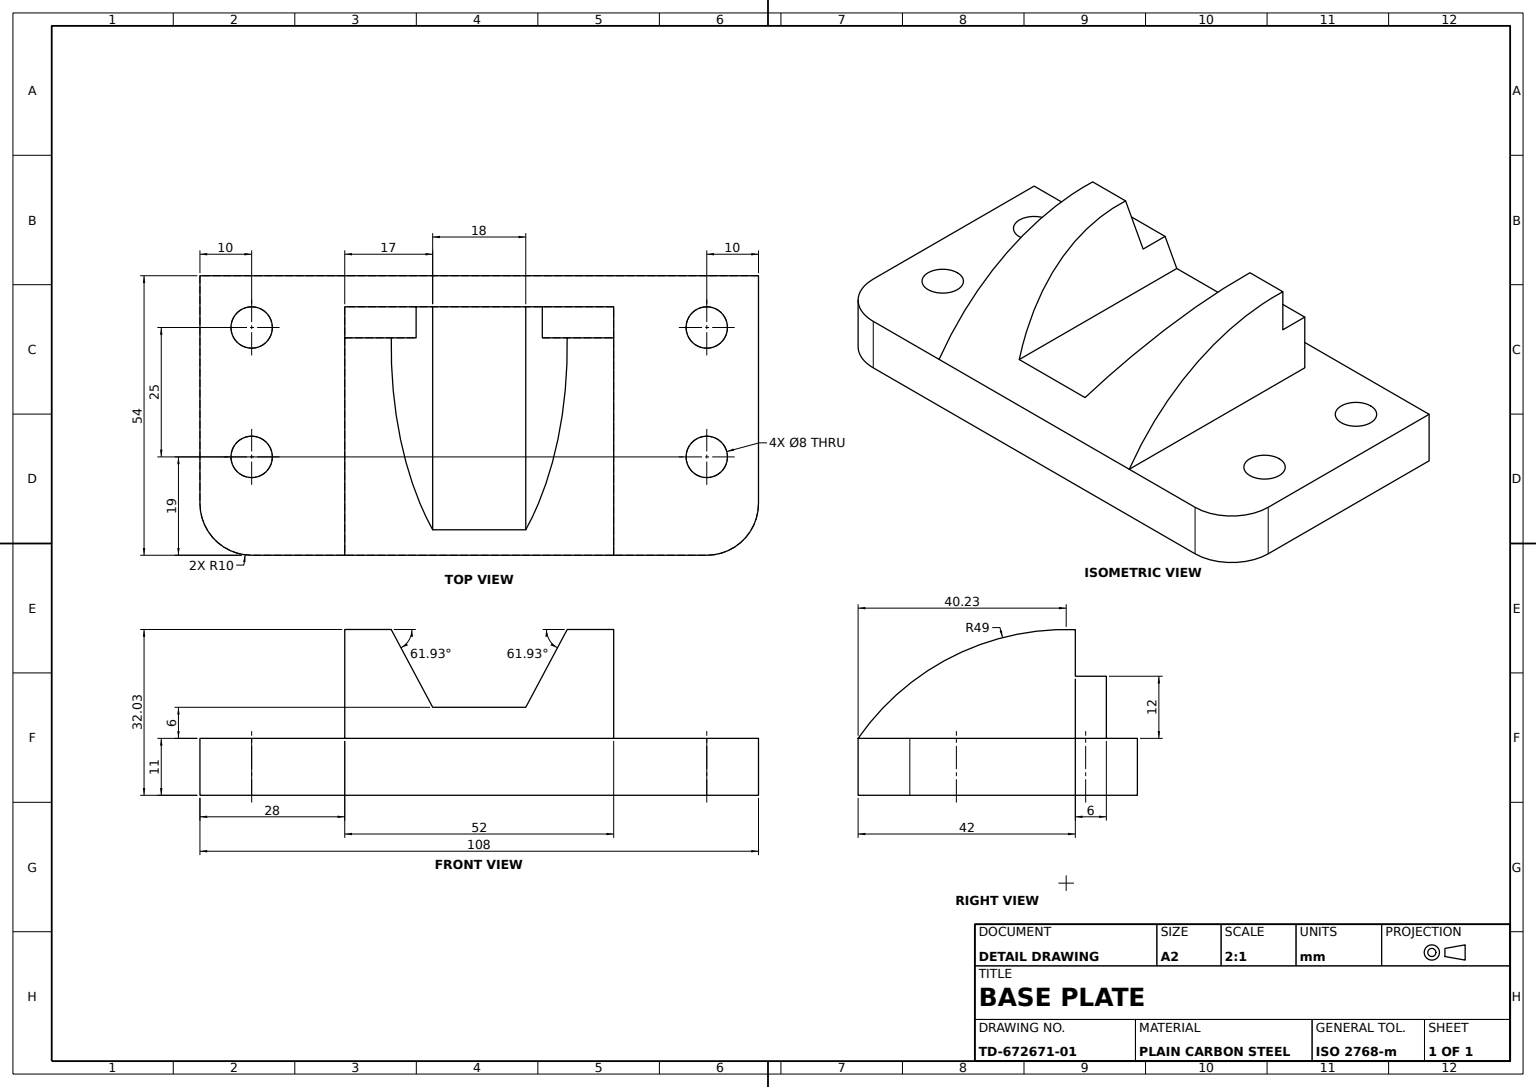
from build123d import *

# Parameters (mm, degrees)
BASE_PLATE_SKETCH_R          = 4
BASE_PLATE_DEPTH             = 11
SADDLE_BLOCK_SKETCH_W        = 52
SADDLE_BLOCK_SKETCH_H        = 48
SADDLE_BLOCK_DEPTH           = 61
SADDLE_ARC_PROFILE_CUT_DEPTH = 61
SADDLE_RELIEF_CUT_DEPTH      = 61


with BuildPart() as part:
    # Base Plate Sketch → Base Plate (new body)
    with BuildSketch(Plane(origin=(0, 0, 0), x_dir=(1, 0, 0), z_dir=(0, 1, 0))):
        with BuildLine():
            Line((-44, -27), (44, -27))
            ThreePointArc((44, -27), (51.071067812, -24.071067812), (54, -17))
            Line((54, -17), (54, 27))
            Line((54, 27), (-54, 27))
            Line((-54, 27), (-54, -17))
            ThreePointArc((-54, -17), (-51.071067812, -24.071067812), (-44, -27))
        make_face()
        with Locations(Location((-44, 17, 0), (0, 0, 270))):
            Circle(BASE_PLATE_SKETCH_R, mode=Mode.SUBTRACT)
        with Locations(Location((-44, -8, 0), (0, 0, 270))):
            Circle(BASE_PLATE_SKETCH_R, mode=Mode.SUBTRACT)
        with Locations(Location((44, 17, 0), (0, 0, 270))):
            Circle(BASE_PLATE_SKETCH_R, mode=Mode.SUBTRACT)
        with Locations(Location((44, -8, 0), (0, 0, 270))):
            Circle(BASE_PLATE_SKETCH_R, mode=Mode.SUBTRACT)
    extrude(amount=BASE_PLATE_DEPTH)

    # Saddle Block Sketch → Saddle Block (add)
    with BuildSketch(Plane(origin=(0, 11, 0), x_dir=(1, 0, 0), z_dir=(0, 1, 0))):
        with Locations((0, -3)):
            Rectangle(SADDLE_BLOCK_SKETCH_W, SADDLE_BLOCK_SKETCH_H)
    extrude(amount=SADDLE_BLOCK_DEPTH)

    # Saddle Arc Profile Sketch → Saddle Arc Profile Cut (cut)
    with BuildSketch(Plane(origin=(26, 0, 0), x_dir=(0, 0, -1), z_dir=(1, 0, 0))):
        with BuildLine():
            Line((15, 23), (15, 32))
            ThreePointArc((15, 32), (-8.67938185, 26.8587637), (-27, 11))
            Line((-27, 11), (-38.885663345, 11))
            Line((-38.885663345, 11), (-38.885663345, 85.95954857))
            Line((-38.885663345, 85.95954857), (45.449794115, 85.95954857))
            Line((45.449794115, 85.95954857), (44.243086456, 28.305738224))
            Line((44.243086456, 28.305738224), (21, 23))
            Line((21, 23), (15, 23))
        make_face()
    extrude(amount=-SADDLE_ARC_PROFILE_CUT_DEPTH, mode=Mode.SUBTRACT)

    # Saddle Relief Sketch → Saddle Relief Cut (cut)
    with BuildSketch(Plane.XY.offset(27)):
        Polygon((-17.016976715, 32.031831341), (17.016976715, 32.031831341), (9, 17), (-9, 17), align=None)
    extrude(amount=-SADDLE_RELIEF_CUT_DEPTH, mode=Mode.SUBTRACT)


solid = part.part
